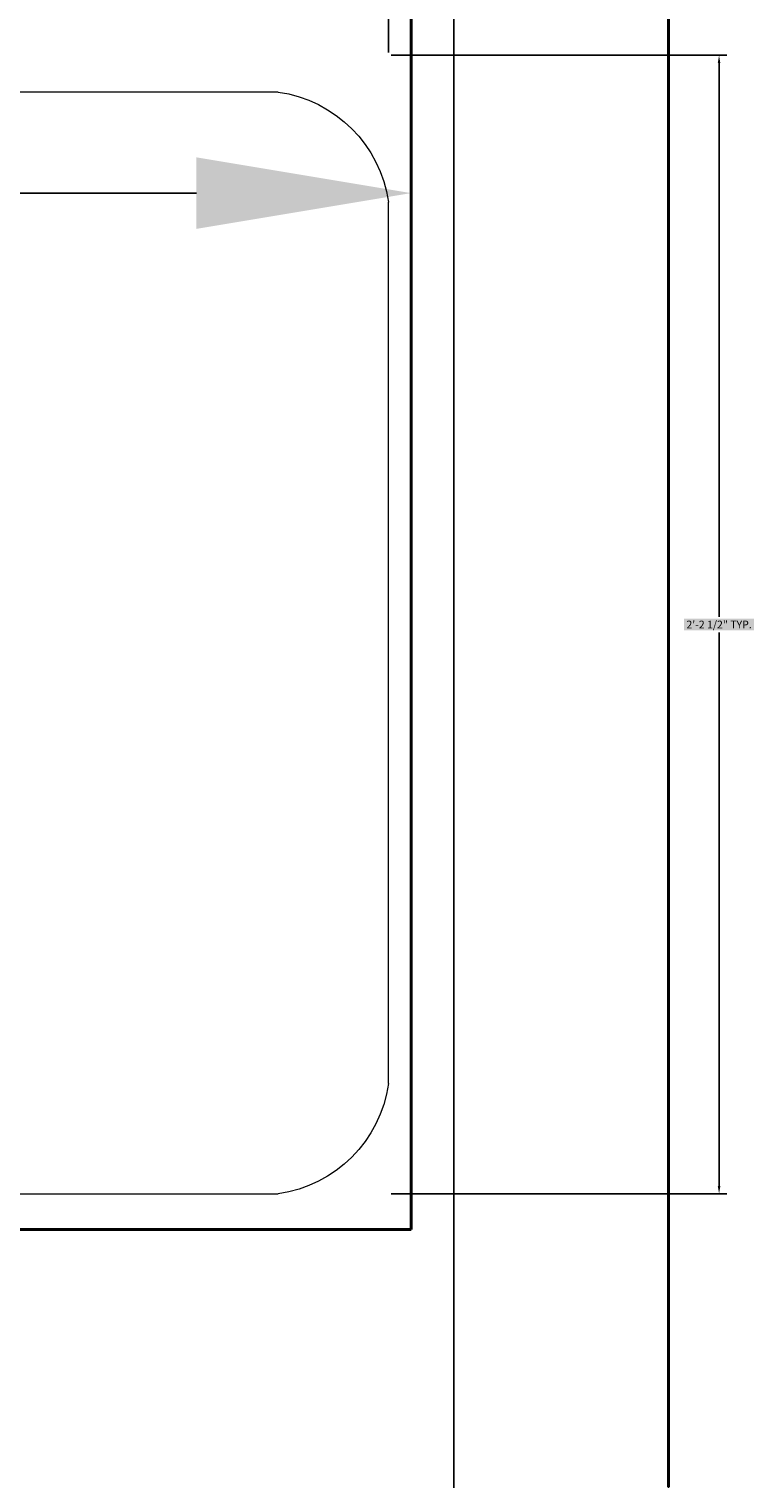
# Model space of a CAD drawing. Units: inches. Extents: x -301 to 715, y -607 to 364.
# Tile 80 of 141: x -61 to -44, y -73 to -39. Entities that reach past the tile are written whole.
import ezdxf

# ---------------------------------------------------------------- set-up
doc = ezdxf.new("R2010")
doc.units = ezdxf.units.IN
doc.header["$MEASUREMENT"] = 0
for name, color, linetype, lineweight in [('A-ANNO-DIMS', 2, 'Continuous', 18), ('A-FURN', 8, 'Continuous', 18), ('A-WALL', 3, 'Continuous', 40)]:
    doc.layers.add(name, color=color, linetype=linetype, lineweight=lineweight)
doc.styles.get("Standard").update_dxf_attribs({"font": 'arial.ttf'})
doc.dimstyles.get("Standard").update_dxf_attribs({"dimtxt": 0.18, "dimasz": 0.18, "dimexe": 0.18, "dimexo": 0.0625, "dimgap": 0.09, "dimtad": 0, "dimtih": 1, "dimtoh": 1, "dimdec": 1, "dimzin": 0, "dimdsep": 46, "dimlunit": 4, "dimtxsty": 'Standard', "dimcen": 0.09, "dimclrd": 3, "dimclre": 4, "dimclrt": 6, "dimadec": 0, "dimazin": 0, "dimtfac": 1, "dimtdec": 1, "dimtofl": 0, "dimtmove": 0, "dimatfit": 3, "dimfxl": 1, "dimtfill": 2, "dimtfillclr": 51, "dimtolj": 1, "dimtzin": 0, "dimarcsym": 0})

# ---------------------------------------------------------------- blocks, each defined once
blk = doc.blocks.new('Desk - 30 x 60 in.')
for p, q in [((-26.999995, 0), (26.999995, 0)), ((29.999995, -3), (29.999995, -27)), ((26.999995, -30), (-26.999995, -30))]:
    blk.add_line(p, q)
for centre, start, end in [((26.499995, -3.5), 8.130102, 81.8699), ((26.499995, -26.5), 278.1301, 351.8699)]:
    blk.add_arc(centre, 3.535534, start, end)
blk = doc.blocks.new('*D57')
at = {"layer": 'A-ANNO-DIMS', "color": 0, "lineweight": -2, "transparency": 16777216}
for p, q in [((-195.603, -67.255), (-195.603, -42.99)), ((-190.603, -43.17), (-126.098, -43.17)), ((-56.603, -43.17), (-121.109, -43.17)), ((-51.603, -67.255), (-51.603, -42.99))]:
    blk.add_line(p, q, dxfattribs=at)
at = {"layer": 'A-ANNO-DIMS', "color": 0, "transparency": 16777216}
for points in [[(-190.603, -42.336), (-190.603, -44.003), (-195.603, -43.17)], [(-56.603, -42.336), (-56.603, -44.003), (-51.603, -43.17)]]:
    blk.add_solid(points, dxfattribs=at)
at = {"layer": 'Defpoints', "color": 0, "transparency": 16777216}
for p in [(-51.603, -43.17), (-195.603, -67.318), (-51.603, -67.318)]:
    blk.add_point(p, dxfattribs=at)
at = {"layer": 'A-ANNO-DIMS', "color": 0, "transparency": 16777216, "insert": (-123.603, -43.17), "char_height": 3, "attachment_point": 5, "bg_fill": 1, "box_fill_scale": 1.25, "bg_fill_color": 51, "bg_fill_transparency": 0}
blk.add_mtext("\\A1;12'", dxfattribs=at)
blk = doc.blocks.new('*D114')
at = {"layer": 'A-ANNO-DIMS', "color": 4, "lineweight": -2, "transparency": 16777216}
for p, q in [((-103.477, -39.895), (-103.477, -32.076)), ((-52.128, -39.895), (-52.128, -32.076))]:
    blk.add_line(p, q, dxfattribs=at)
at = {"layer": 'A-ANNO-DIMS', "color": 3, "lineweight": -2, "transparency": 16777216}
for p, q in [((-103.297, -32.256), (-79.024, -32.256)), ((-52.308, -32.256), (-76.581, -32.256))]:
    blk.add_line(p, q, dxfattribs=at)
at = {"layer": 'A-ANNO-DIMS', "color": 3, "transparency": 16777216}
for points in [[(-103.297, -32.226), (-103.297, -32.286), (-103.477, -32.256)], [(-52.308, -32.226), (-52.308, -32.286), (-52.128, -32.256)]]:
    blk.add_solid(points, dxfattribs=at)
at = {"layer": 'Defpoints', "color": 0, "transparency": 16777216}
for p in [(-52.128, -32.256), (-103.477, -39.958), (-52.128, -39.958)]:
    blk.add_point(p, dxfattribs=at)
at = {"layer": 'A-ANNO-DIMS', "color": 6, "transparency": 16777216, "insert": (-77.803, -32.256), "char_height": 0.18, "attachment_point": 5, "bg_fill": 1, "box_fill_scale": 1.25, "bg_fill_color": 51, "bg_fill_transparency": 0}
blk.add_mtext('\\A1;DESK 4\'-3 1/2" TYP.', dxfattribs=at)
blk = doc.blocks.new('*D115')
at = {"layer": 'A-ANNO-DIMS', "color": 4, "lineweight": -2, "transparency": 16777216}
for p, q in [((-52.066, -39.958), (-44.246, -39.958)), ((-52.066, -66.488), (-44.246, -66.488))]:
    blk.add_line(p, q, dxfattribs=at)
at = {"layer": 'A-ANNO-DIMS', "color": 3, "lineweight": -2, "transparency": 16777216}
for p, q in [((-44.426, -40.138), (-44.426, -53.04)), ((-44.426, -66.308), (-44.426, -53.406))]:
    blk.add_line(p, q, dxfattribs=at)
at = {"layer": 'A-ANNO-DIMS', "color": 3, "transparency": 16777216}
for points in [[(-44.456, -40.138), (-44.396, -40.138), (-44.426, -39.958)], [(-44.456, -66.308), (-44.396, -66.308), (-44.426, -66.488)]]:
    blk.add_solid(points, dxfattribs=at)
at = {"layer": 'Defpoints', "color": 0, "transparency": 16777216}
for p in [(-52.128, -39.958), (-52.128, -66.488), (-44.426, -66.488)]:
    blk.add_point(p, dxfattribs=at)
at = {"layer": 'A-ANNO-DIMS', "color": 6, "transparency": 16777216, "insert": (-44.426, -53.223), "char_height": 0.18, "attachment_point": 5, "bg_fill": 1, "box_fill_scale": 1.25, "bg_fill_color": 51, "bg_fill_transparency": 0}
blk.add_mtext('\\A1;2\'-2 1/2" TYP.', dxfattribs=at)
blk = doc.blocks.new('*D151')
at = {"layer": 'A-ANNO-DIMS', "color": 4, "lineweight": -2, "transparency": 16777216}
for p, q in [((-204.603, -223.755), (-204.603, 359.612)), ((-45.603, -214.755), (-45.603, 359.612))]:
    blk.add_line(p, q, dxfattribs=at)
at = {"layer": 'A-ANNO-DIMS', "color": 3, "lineweight": -2, "transparency": 16777216}
for p, q in [((-204.423, 359.432), (-125.494, 359.432)), ((-45.783, 359.432), (-124.713, 359.432))]:
    blk.add_line(p, q, dxfattribs=at)
at = {"layer": 'A-ANNO-DIMS', "color": 3, "transparency": 16777216}
for points in [[(-204.423, 359.462), (-204.423, 359.402), (-204.603, 359.432)], [(-45.783, 359.462), (-45.783, 359.402), (-45.603, 359.432)]]:
    blk.add_solid(points, dxfattribs=at)
at = {"layer": 'Defpoints', "color": 0, "transparency": 16777216}
for p in [(-45.603, 359.432), (-45.603, -214.818), (-204.603, -223.818)]:
    blk.add_point(p, dxfattribs=at)
at = {"layer": 'A-ANNO-DIMS', "color": 6, "transparency": 16777216, "insert": (-125.103, 359.432), "char_height": 0.18, "attachment_point": 5, "bg_fill": 1, "box_fill_scale": 1.25, "bg_fill_color": 51, "bg_fill_transparency": 0}
blk.add_mtext('\\A1;13\'-3"', dxfattribs=at)
blk = doc.blocks.new('*D158')
at = {"layer": 'A-ANNO-DIMS', "color": 4, "lineweight": -2, "transparency": 16777216}
for p, q in [((-122.603, 221.62), (-122.603, -296.865)), ((-50.603, 221.62), (-50.603, -296.865))]:
    blk.add_line(p, q, dxfattribs=at)
at = {"layer": 'A-ANNO-DIMS', "color": 3, "lineweight": -2, "transparency": 16777216}
for p, q in [((-122.423, -296.685), (-86.933, -296.685)), ((-50.783, -296.685), (-86.274, -296.685))]:
    blk.add_line(p, q, dxfattribs=at)
at = {"layer": 'A-ANNO-DIMS', "color": 3, "transparency": 16777216}
for points in [[(-122.423, -296.655), (-122.423, -296.715), (-122.603, -296.685)], [(-50.783, -296.655), (-50.783, -296.715), (-50.603, -296.685)]]:
    blk.add_solid(points, dxfattribs=at)
at = {"layer": 'Defpoints', "color": 0, "transparency": 16777216}
for p in [(-122.603, 221.682), (-50.603, 221.682), (-50.603, -296.685)]:
    blk.add_point(p, dxfattribs=at)
at = {"layer": 'A-ANNO-DIMS', "color": 6, "transparency": 16777216, "insert": (-86.603, -296.685), "char_height": 0.18, "attachment_point": 5, "bg_fill": 1, "box_fill_scale": 1.25, "bg_fill_color": 51, "bg_fill_transparency": 0}
blk.add_mtext('\\A1;6\'-0"', dxfattribs=at)

msp = doc.modelspace()

# ---------------------------------------------------------------- linework, layer by layer
at = {"layer": 'A-WALL'}
for p, q in [((-51.603, -67.318), (-51.603, 25.682)), ((-45.603, -73.318), (-45.603, 25.682)), ((-51.603, -64.915), (-51.603, -63.165)), ((-195.603, -67.318), (-51.603, -67.318))]:
    msp.add_line(p, q, dxfattribs=at)

# ---------------------------------------------------------------- block references
at = {"layer": 'A-FURN', "xscale": -0.8558048107780498, "yscale": 0.8558048107780498, "zscale": 0.8558048107780498, "rotation": 180}
msp.add_blockref('Desk - 30 x 60 in.', (-77.803, -66.488), dxfattribs=at)

# ---------------------------------------------------------------- dimensions: what is measured, and where the dimension line sits
at = {"layer": 'A-ANNO-DIMS'}
for base, p1, p2, override, picture, middle in [((-45.603, 359.432), (-204.603, -223.818), (-45.603, -214.818), {"dimdec": 1, "dimlfac": 1, "dimrnd": 0, "dimzin": 1, "dimdsep": 46, "dimlunit": 4, "dimfrac": 2}, '*D151', (-125.103, 359.432)), ((-50.603, -296.685), (-122.603, 221.682), (-50.603, 221.682), {"dimdec": 1, "dimlfac": 1, "dimrnd": 0, "dimzin": 1, "dimdsep": 46, "dimlunit": 4, "dimfrac": 2}, '*D158', (-86.603, -296.685)), ((-51.603, -43.17), (-195.603, -67.318), (-51.603, -67.318), {"dimtxt": 3, "dimasz": 5, "dimclrd": 0, "dimclre": 0, "dimclrt": 0}, '*D57', (-123.603, -43.17))]:
    dim = msp.add_linear_dim(base=base, p1=p1, p2=p2, dimstyle='Standard', override=override, dxfattribs=at)
    dim.commit()
    dim.dimension.update_dxf_attribs({"geometry": picture, "text_midpoint": middle})
dim = msp.add_linear_dim(base=(-52.128, -32.256), p1=(-103.477, -39.958), p2=(-52.128, -39.958), text='DESK <> TYP.', dimstyle='Standard', override={"dimdec": 1, "dimlfac": 1, "dimrnd": 0, "dimzin": 1, "dimdsep": 46, "dimlunit": 4, "dimfrac": 2}, dxfattribs=at)
dim.commit()
dim.dimension.update_dxf_attribs({"geometry": '*D114', "text_midpoint": (-77.803, -32.256)})
dim = msp.add_linear_dim(base=(-44.426, -66.488), p1=(-52.128, -39.958), p2=(-52.128, -66.488), angle=270, text='<> TYP.', dimstyle='Standard', override={"dimdec": 1, "dimlfac": 1, "dimrnd": 0, "dimzin": 1, "dimdsep": 46, "dimlunit": 4, "dimfrac": 2}, dxfattribs=at)
dim.commit()
dim.dimension.update_dxf_attribs({"geometry": '*D115', "text_midpoint": (-44.426, -53.223)})

doc.saveas('drawing.dxf')
